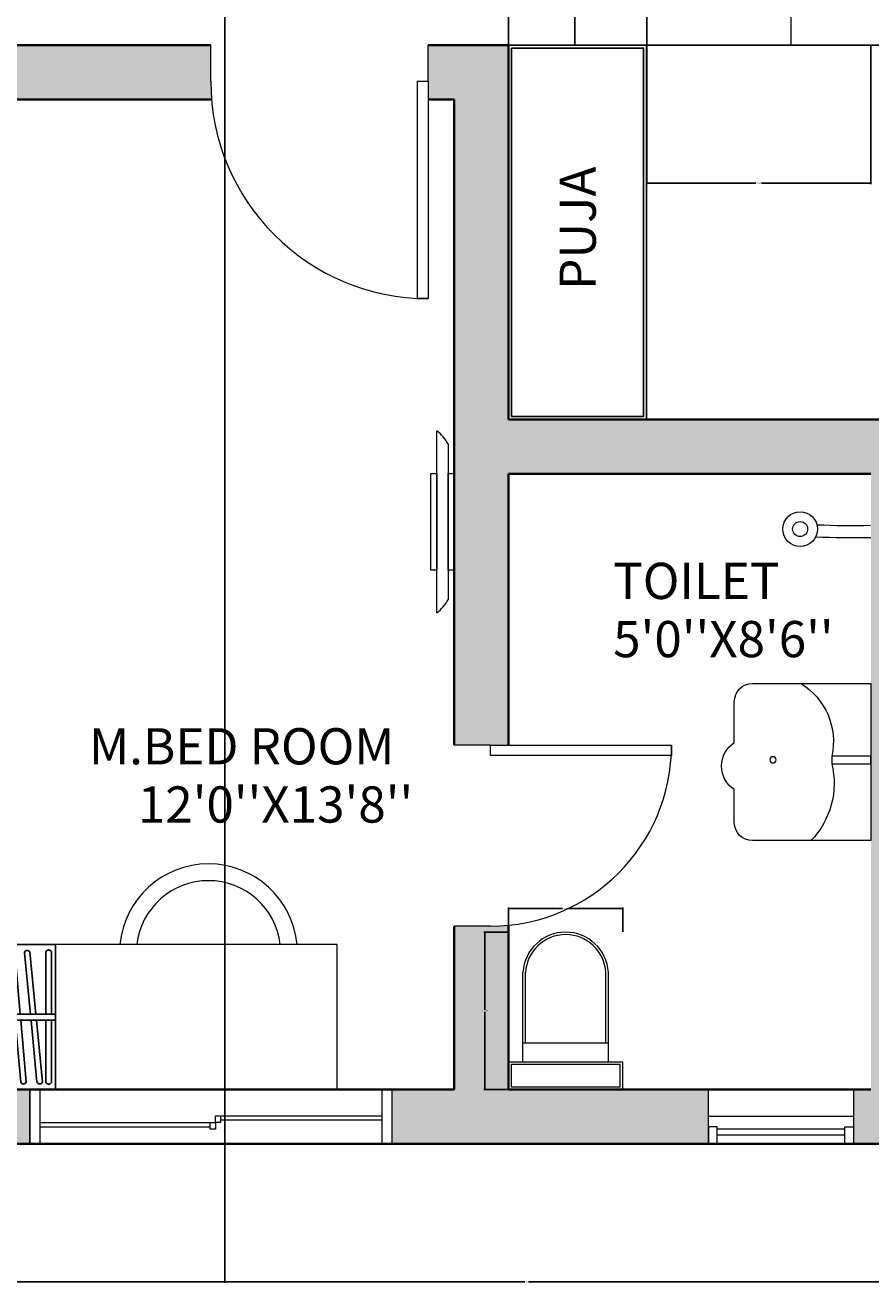
# Model space of a CAD drawing. Units: inches. Extents: x 1789 to 2841, y 3180 to 3702.
# Tile 3 of 14: x 2041 to 2181, y 3180 to 3388. Entities that reach past the tile are written whole.
import ezdxf

# ---------------------------------------------------------------- set-up
doc = ezdxf.new("R2010")
doc.units = ezdxf.units.IN
doc.header["$MEASUREMENT"] = 0
for name, color, linetype, lineweight in [('A-ANNO-DIMS', 2, 'Continuous', 18), ('A-AREA-IDEN', 7, 'Continuous', 18), ('A-EQPM', 8, 'Continuous', 18), ('A-FLOR-CASE', 34, 'Continuous', 25), ('A-FLOR-FIXT', 9, 'Continuous', 18), ('A-WALL', 40, 'Continuous', 35), ('A-WALL-PATT', 252, 'Continuous', 13), ('DORS', 70, 'Continuous', 18), ('FURNITURE', 34, 'Continuous', 18), ('WINDOWS', 130, 'Continuous', 18)]:
    doc.layers.add(name, color=color, linetype=linetype, lineweight=lineweight)
doc.styles.get("Standard").update_dxf_attribs({"font": 'arial.ttf'})
doc.dimstyles.get("Standard").update_dxf_attribs({"dimtxt": 0.18, "dimasz": 0.18, "dimexe": 0.18, "dimexo": 0.0625, "dimgap": 0.09, "dimtad": 0, "dimtih": 1, "dimtoh": 1, "dimdec": 0, "dimzin": 0, "dimdsep": 46, "dimlunit": 3, "dimtxsty": 'Standard', "dimcen": 0.09, "dimadec": 0, "dimazin": 0, "dimtfac": 1, "dimtdec": 0, "dimtofl": 0, "dimtmove": 0, "dimatfit": 3, "dimfxl": 1, "dimtolj": 1, "dimtzin": 0, "dimarcsym": 0})

# ---------------------------------------------------------------- blocks, each defined once
blk = doc.blocks.new('CUBOARD')
for p, q in [((2183.73, 3646.16), (2183.73, 3568.16)), ((2184.71, 3646.16), (2184.71, 3568.16))]:
    blk.add_line(p, q)
blk.add_lwpolyline([(2172.23, 3646.16), (2196.23, 3646.16), (2196.23, 3568.16), (2172.23, 3568.16)], close=True)
for points in [[(2183.69, 3644.46), (2173.95, 3643.51)], [(2195.39, 3645.6), (2184.67, 3644.55)], [(2184.76, 3643.66), (2195.54, 3644.71)], [(2195.78, 3645.16), (2195.78, 3645.18)], [(2183.73, 3641.98), (2173.93, 3641.98)], [(2173.97, 3642.61), (2183.78, 3643.57)], [(2195.47, 3641.98), (2184.71, 3641.98)], [(2173.86, 3641.08), (2183.73, 3641.08)], [(2183.76, 3639.46), (2173.96, 3640.08)], [(2184.71, 3641.08), (2195.53, 3641.08)], [(2195.82, 3641.5), (2195.82, 3641.53)], [(2173.84, 3639.19), (2183.7, 3638.57)], [(2184.68, 3638.5), (2195.46, 3637.81)], [(2195.45, 3638.71), (2184.74, 3639.4)], [(2195.77, 3638.22), (2195.78, 3638.24)], [(2173.83, 3635.92), (2183.73, 3635.92)], [(2183.73, 3636.82), (2173.9, 3636.82)], [(2195.43, 3636.82), (2184.71, 3636.82)], [(2184.71, 3635.92), (2195.5, 3635.92)], [(2195.78, 3636.35), (2195.78, 3636.37)], [(2173.81, 3633.34), (2183.73, 3633.34)], [(2183.73, 3634.24), (2173.88, 3634.24)], [(2195.42, 3634.24), (2184.71, 3634.24)], [(2184.71, 3633.34), (2195.48, 3633.34)], [(2195.77, 3633.77), (2195.77, 3633.79)], [(2183.73, 3631.66), (2173.86, 3631.66)], [(2195.4, 3631.66), (2184.71, 3631.66)], [(2195.75, 3631.19), (2195.75, 3631.21)], [(2173.8, 3630.76), (2183.73, 3630.76)], [(2183.73, 3629.08), (2173.85, 3629.08)], [(2184.71, 3630.76), (2195.47, 3630.76)], [(2195.38, 3629.08), (2184.71, 3629.08)], [(2173.78, 3628.19), (2183.73, 3628.19)], [(2183.8, 3626.57), (2173.93, 3627.31)], [(2184.71, 3628.19), (2195.45, 3628.19)], [(2195.73, 3628.61), (2195.73, 3628.63)], [(2173.79, 3626.43), (2183.74, 3625.68)], [(2184.71, 3625.61), (2195.4, 3624.81)], [(2195.4, 3625.7), (2184.78, 3626.5)], [(2195.72, 3625.21), (2195.72, 3625.23)], [(2173.75, 3623.03), (2183.73, 3623.03)], [(2183.73, 3623.92), (2173.81, 3623.92)], [(2195.35, 3623.92), (2184.71, 3623.92)], [(2184.71, 3623.03), (2195.42, 3623.03)], [(2195.7, 3623.45), (2195.7, 3623.48)], [(2183.73, 3621.34), (2173.8, 3621.34)], [(2195.33, 3621.34), (2184.71, 3621.34)], [(2195.68, 3620.87), (2195.68, 3620.9)], [(2173.73, 3620.45), (2183.73, 3620.45)], [(2183.67, 3618.69), (2173.75, 3617.93)], [(2195.22, 3619.57), (2184.65, 3618.76)], [(2184.71, 3620.45), (2195.4, 3620.45)], [(2184.71, 3617.87), (2195.35, 3618.68)], [(2195.6, 3619.13), (2195.6, 3619.15)], [(2173.75, 3617.03), (2183.74, 3617.8)], [(2173.7, 3615.29), (2183.73, 3615.29)], [(2183.73, 3616.19), (2173.77, 3616.19)], [(2195.3, 3616.19), (2184.71, 3616.19)], [(2184.71, 3615.29), (2195.37, 3615.29)], [(2195.65, 3615.71), (2195.65, 3615.74)], [(2173.68, 3612.71), (2183.73, 3612.71)], [(2183.73, 3613.61), (2173.75, 3613.61)], [(2195.28, 3613.61), (2184.71, 3613.61)], [(2184.71, 3612.71), (2195.35, 3612.71)], [(2195.63, 3613.14), (2195.63, 3613.16)], [(2173.67, 3611.18), (2183.69, 3610.23)], [(2183.78, 3611.12), (2173.82, 3612.07)], [(2195.26, 3610.03), (2184.75, 3611.03)], [(2183.72, 3608.42), (2173.71, 3608.13)], [(2184.67, 3610.14), (2195.24, 3609.13)], [(2195.23, 3608.76), (2184.7, 3608.45)], [(2195.56, 3609.53), (2195.57, 3609.55)], [(2195.6, 3608.3), (2195.6, 3608.32)], [(2173.66, 3607.23), (2183.75, 3607.53)], [(2184.73, 3607.55), (2195.33, 3607.87)], [(2173.63, 3604.98), (2183.73, 3604.98)], [(2183.73, 3605.87), (2173.7, 3605.87)], [(2195.23, 3605.87), (2184.71, 3605.87)], [(2184.71, 3604.98), (2195.3, 3604.98)], [(2195.58, 3605.4), (2195.58, 3605.42)], [(2173.61, 3602.4), (2183.73, 3602.4)], [(2183.73, 3603.29), (2173.68, 3603.29)], [(2195.22, 3603.29), (2184.71, 3603.29)], [(2184.71, 3602.4), (2195.28, 3602.4)], [(2195.57, 3602.82), (2195.57, 3602.84)], [(2183.73, 3600.71), (2173.67, 3600.71)], [(2195.2, 3600.71), (2184.71, 3600.71)], [(2195.55, 3600.24), (2195.55, 3600.27)], [(2173.6, 3599.82), (2183.73, 3599.82)], [(2183.73, 3598.13), (2173.65, 3598.13)], [(2184.71, 3599.82), (2195.27, 3599.82)], [(2195.18, 3598.13), (2184.71, 3598.13)], [(2173.58, 3597.24), (2183.73, 3597.24)], [(2183.77, 3595.62), (2173.68, 3596.25)], [(2184.71, 3597.24), (2195.25, 3597.24)], [(2195.53, 3597.66), (2195.53, 3597.69)], [(2173.56, 3595.36), (2183.71, 3594.72)], [(2184.69, 3594.66), (2195.19, 3594)], [(2195.18, 3594.9), (2184.74, 3595.55)], [(2195.5, 3594.4), (2195.5, 3594.43)], [(2173.55, 3592.08), (2183.73, 3592.08)], [(2183.73, 3592.98), (2173.62, 3592.98)], [(2195.15, 3592.98), (2184.71, 3592.98)], [(2184.71, 3592.08), (2195.22, 3592.08)], [(2195.5, 3592.5), (2195.5, 3592.53)], [(2173.57, 3590.49), (2183.74, 3589.59)], [(2183.73, 3590.49), (2173.72, 3591.37)], [(2195.17, 3589.47), (2184.71, 3590.4)], [(2184.71, 3589.5), (2195.16, 3588.58)], [(2183.73, 3587.82), (2173.58, 3587.82)], [(2195.12, 3587.82), (2184.71, 3587.82)], [(2195.48, 3588.97), (2195.48, 3589)], [(2173.51, 3586.92), (2183.73, 3586.92)], [(2194.84, 3586.83), (2184.58, 3585.23)], [(2184.71, 3586.92), (2195.19, 3586.92)], [(2184.71, 3584.34), (2195.04, 3585.95)], [(2195.26, 3586.41), (2195.25, 3586.44)], [(2195.47, 3587.35), (2195.47, 3587.37)], [(2183.61, 3585.08), (2173.56, 3583.51)], [(2173.63, 3582.62), (2183.75, 3584.19)], [(2173.48, 3581.77), (2183.73, 3581.77)], [(2183.73, 3582.66), (2173.55, 3582.66)], [(2195.08, 3582.66), (2184.71, 3582.66)], [(2184.71, 3581.77), (2195.15, 3581.77)], [(2195.43, 3582.19), (2195.43, 3582.21)], [(2173.46, 3579.19), (2183.73, 3579.19)], [(2183.73, 3580.08), (2173.53, 3580.08)], [(2195.07, 3580.08), (2184.71, 3580.08)], [(2184.71, 3579.19), (2195.14, 3579.19)], [(2195.42, 3579.61), (2195.42, 3579.63)], [(2183.73, 3577.5), (2173.52, 3577.5)], [(2195.05, 3577.5), (2184.71, 3577.5)], [(2195.4, 3577.03), (2195.4, 3577.05)], [(2173.45, 3576.61), (2183.73, 3576.61)], [(2194.92, 3575.81), (2184.64, 3574.92)], [(2184.71, 3576.61), (2195.12, 3576.61)], [(2184.71, 3574.03), (2195.06, 3574.93)], [(2195.31, 3575.37), (2195.31, 3575.4)], [(2183.66, 3574.84), (2173.46, 3573.95)], [(2173.47, 3573.05), (2183.74, 3573.94)], [(2194.88, 3573.34), (2184.63, 3572.34)], [(2195.28, 3572.91), (2195.27, 3572.93)], [(2183.65, 3572.24), (2173.45, 3571.25)], [(2173.47, 3570.35), (2183.74, 3571.35)], [(2184.71, 3571.45), (2195.04, 3572.46)], [(2173.4, 3568.87), (2183.73, 3568.87)], [(2183.73, 3569.77), (2173.47, 3569.77)], [(2195, 3569.77), (2184.71, 3569.77)], [(2184.71, 3568.87), (2195.07, 3568.87)], [(2195.35, 3569.29), (2195.35, 3569.32)]]:
    blk.add_lwpolyline(points)
for centre, start, end in [((2195.31, 3645.13), 7.0195, 80.386), ((2195.31, 3645.13), 299.464, 4.1032), ((2174.06, 3641.52), 105.1753, 246.0974), ((2174.12, 3643.06), 110.7367, 251.6587), ((2195.34, 3641.52), 1.4582, 74.8247), ((2174.06, 3639.62), 101.5232, 242.4452), ((2195.34, 3641.52), 293.9026, 358.5418), ((2195.3, 3638.26), 357.8061, 71.1726), ((2195.3, 3638.26), 290.2505, 354.8897), ((2174.02, 3636.36), 105.1753, 246.0974), ((2195.31, 3636.36), 1.4582, 74.8247), ((2195.31, 3636.36), 293.9026, 358.5418), ((2174.01, 3633.78), 105.1753, 246.0974), ((2195.29, 3633.78), 1.4582, 74.8247), ((2195.29, 3633.78), 293.9026, 358.5418), ((2173.99, 3631.2), 105.1753, 246.0974), ((2195.27, 3631.2), 1.4582, 74.8247), ((2195.27, 3631.2), 293.9026, 358.5418), ((2173.97, 3628.62), 105.1753, 246.0974), ((2195.26, 3628.62), 1.4582, 74.8247), ((2174.02, 3626.85), 100.888, 241.81), ((2195.26, 3628.62), 293.9026, 358.5418), ((2195.24, 3625.25), 357.1709, 70.5374), ((2195.24, 3625.25), 289.6153, 354.2545), ((2173.94, 3623.46), 105.1753, 246.0974), ((2195.22, 3623.46), 1.4582, 74.8247), ((2195.22, 3623.46), 293.9026, 358.5418), ((2173.92, 3620.88), 105.1753, 246.0974), ((2195.21, 3620.88), 1.4582, 74.8247), ((2195.21, 3620.88), 293.9026, 358.5418), ((2195.13, 3619.1), 5.8369, 79.2034), ((2195.13, 3619.1), 298.2814, 2.9206), ((2173.9, 3617.48), 109.5541, 250.4761), ((2173.89, 3615.73), 105.1753, 246.0974), ((2195.17, 3615.73), 1.4582, 74.8247), ((2195.17, 3615.73), 293.9026, 358.5418), ((2173.87, 3613.15), 105.1753, 246.0974), ((2195.16, 3613.15), 1.4582, 74.8247), ((2195.16, 3613.15), 293.9026, 358.5418), ((2173.9, 3611.6), 99.7479, 240.6699), ((2195.12, 3608.3), 3.1408, 76.5073), ((2195.09, 3609.58), 288.4752, 353.1144), ((2195.09, 3609.58), 356.0307, 69.3973), ((2195.12, 3608.3), 295.5853, 0.2245), ((2173.84, 3607.67), 106.858, 247.78), ((2173.82, 3605.41), 105.1753, 246.0974), ((2195.11, 3605.41), 1.4582, 74.8247), ((2195.11, 3605.41), 293.9026, 358.5418), ((2173.81, 3602.83), 105.1753, 246.0974), ((2195.09, 3602.83), 1.4582, 74.8247), ((2195.09, 3602.83), 293.9026, 358.5418), ((2173.79, 3600.25), 105.1753, 246.0974), ((2195.08, 3600.25), 1.4582, 74.8247), ((2195.08, 3600.25), 293.9026, 358.5418), ((2173.77, 3597.67), 105.1753, 246.0974), ((2195.06, 3597.67), 1.4582, 74.8247), ((2173.78, 3595.78), 101.566, 242.4881), ((2195.06, 3597.67), 293.9026, 358.5418), ((2195.02, 3594.44), 357.8489, 71.2154), ((2195.02, 3594.44), 290.2933, 354.9325), ((2173.74, 3592.52), 105.1753, 246.0974), ((2195.03, 3592.52), 1.4582, 74.8247), ((2195.03, 3592.52), 293.9026, 358.5418), ((2173.8, 3590.9), 100.1162, 241.0382), ((2173.71, 3587.36), 105.1753, 246.0974), ((2194.99, 3587.36), 1.4582, 74.8247), ((2195.01, 3589.03), 288.8435, 353.4827), ((2195.01, 3589.03), 356.399, 69.7655), ((2194.79, 3586.35), 10.3063, 83.6728), ((2194.79, 3586.35), 302.7507, 7.3899), ((2194.99, 3587.36), 293.9026, 358.5418), ((2173.75, 3583.08), 114.0234, 254.9455), ((2173.67, 3582.2), 105.1753, 246.0974), ((2194.96, 3582.2), 1.4582, 74.8247), ((2194.96, 3582.2), 293.9026, 358.5418), ((2173.66, 3579.62), 105.1753, 246.0974), ((2194.94, 3579.62), 1.4582, 74.8247), ((2194.94, 3579.62), 293.9026, 358.5418), ((2173.64, 3577.04), 105.1753, 246.0974), ((2194.93, 3577.04), 1.4582, 74.8247), ((2194.93, 3577.04), 293.9026, 358.5418), ((2194.83, 3575.34), 6.4142, 79.7807), ((2194.83, 3575.34), 298.8587, 3.4979), ((2173.63, 3573.5), 110.1314, 251.0534), ((2194.8, 3572.87), 7.0476, 80.4142), ((2194.8, 3572.87), 299.4921, 4.1313), ((2173.62, 3570.8), 110.7648, 251.6868), ((2173.59, 3569.31), 105.1753, 246.0974), ((2194.88, 3569.31), 1.4582, 74.8247), ((2194.88, 3569.31), 293.9026, 358.5418)]:
    blk.add_arc(centre, 0.476, start, end)
blk = doc.blocks.new('KIKI')
blk.add_lwpolyline([(2076.233, 3621.086), (2067.627, 3621.086), (2067.627, 3604.375), (2076.233, 3604.375)], close=True)
for radius, start, end in [(5.285, 95.30288, 264.69712), (4.285, 96.54542, 263.45458)]:
    blk.add_arc((2068.115, 3613.452), radius, start, end)
blk = doc.blocks.new('HYJ')
for p, q in [((2236.02, 3650.77), (2262.74, 3650.77)), ((2236.02, 3650.11), (2262.74, 3650.11)), ((2206.12, 3649.67), (2234.3, 3649.67)), ((2206.12, 3649), (2234.3, 3649))]:
    blk.add_line(p, q)
for points in [[(2204.43, 3646.16), (2264.43, 3646.16), (2264.43, 3655.16), (2204.43, 3655.16)], [(2204.43, 3655.16), (2206.12, 3655.16), (2206.12, 3646.16), (2204.43, 3646.16)], [(2264.43, 3655.16), (2262.74, 3655.16), (2262.74, 3646.16), (2264.43, 3646.16)], [(2235.16, 3650.77), (2236.02, 3650.77), (2236.02, 3649.67), (2235.16, 3649.67)], [(2234.3, 3649.67), (2235.16, 3649.67), (2235.16, 3648.56), (2234.3, 3648.56)]]:
    blk.add_lwpolyline(points, close=True)
blk = doc.blocks.new('*U9')
for p, q in [((0, 0), (0, -6)), ((36, 0), (36, -6))]:
    blk.add_line(p, q)
blk.add_lwpolyline([(0, 0), (0, 36), (1.75, 36), (1.75, 0)], close=True)
blk.add_arc((0, 0), 36, 0, 90)
blk = doc.blocks.new('GTGTG')
for points in [[(2266.82, 3646.16), (2282.82, 3646.16), (2282.82, 3645.14), (2266.82, 3645.14)], [(2266.82, 3643.29), (2282.82, 3643.29), (2282.82, 3642.27), (2266.82, 3642.27)]]:
    blk.add_lwpolyline(points, close=True)
for points in [[(2261.92, 3645.14), (2287.72, 3645.14)], [(2289.9, 3643.29), (2259.74, 3643.29)]]:
    blk.add_lwpolyline(points)
for centre, start, end in [((2265.21, 3639.05), 118.4184, 142.2436), ((2284.43, 3639.05), 37.7564, 61.5816)]:
    blk.add_arc(centre, 6.92, start, end)
blk = doc.blocks.new('*U10')
for p, q in [((0, 0), (0, -6)), ((30, 0), (30, -6))]:
    blk.add_line(p, q)
blk.add_lwpolyline([(0, 0), (0, 30), (1.75, 30), (1.75, 0)], close=True)
blk.add_arc((0, 0), 30, 0, 90)
blk = doc.blocks.new('HY')
for p, q in [((2053.67, 3653.75), (2074.8, 3653.75)), ((2053.67, 3652.75), (2074.8, 3652.75)), ((2052.23, 3650.66), (2076.23, 3650.66))]:
    blk.add_line(p, q)
for points in [[(2076.23, 3646.16), (2052.23, 3646.16), (2052.23, 3655.16), (2076.23, 3655.16)], [(2052.23, 3655.16), (2053.67, 3655.16), (2053.67, 3652.35), (2052.23, 3652.35)], [(2076.23, 3655.16), (2074.8, 3655.16), (2074.8, 3652.35), (2076.23, 3652.35)]]:
    blk.add_lwpolyline(points, close=True)
blk = doc.blocks.new('GT')
for p, q in [((2141.38, 3640.15), (2141.38, 3620.49)), ((2160.08, 3640.15), (2160.08, 3620.49)), ((2141.38, 3636.04), (2160.08, 3636.04)), ((2141.93, 3636.04), (2141.93, 3620.49)), ((2159.53, 3636.04), (2159.53, 3620.49))]:
    blk.add_line(p, q)
for points in [[(2163.23, 3646.16), (2138.23, 3646.16), (2138.23, 3640.15), (2163.23, 3640.15)], [(2162.68, 3645.61), (2138.78, 3645.61), (2138.78, 3640.7), (2162.68, 3640.7)]]:
    blk.add_lwpolyline(points, close=True)
for radius in [8.82, 9.37]:
    blk.add_arc((2150.73, 3621.09), radius, 183.6546, 356.3454)
blk = doc.blocks.new('TYTY')
for p, q in [((2104.84, 3607.68), (2085.23, 3607.68)), ((2085.23, 3607.68), (2085.23, 3581.66)), ((2107.84, 3597.9), (2107.84, 3604.68)), ((2107.84, 3584.66), (2107.84, 3590.13)), ((2085.23, 3581.66), (2104.84, 3581.66))]:
    blk.add_line(p, q)
blk.add_lwpolyline([(2085.23, 3595.66), (2091.71, 3595.66), (2091.71, 3594.41), (2085.23, 3594.41)], close=True)
blk.add_circle((2101.42, 3595.04), 0.517)
for centre, radius, start, end in [((2102.58, 3598.14), 11.14, 121.1396, 192.8397), ((2104.84, 3604.68), 3, 0, 90), ((2105.34, 3594.01), 4.62, 302.7804, 57.2196), ((2104.89, 3591.14), 13.58, 166.0641, 224.2681), ((2104.84, 3584.66), 3, 270, 0)]:
    blk.add_arc(centre, radius, start, end)
blk = doc.blocks.new('SOFA')
for p, q in [((2185.57, 3479.13), (2185.57, 3482.99)), ((2185.57, 3482.99), (2290.09, 3482.99)), ((2290.09, 3482.99), (2290.09, 3460.33)), ((2159.93, 3439.46), (2194.03, 3439.46)), ((2226.79, 3388.76), (2226.79, 3418.07)), ((2260.29, 3388.76), (2260.29, 3418.07)), ((2310.14, 3409.22), (2310.14, 3394.77))]:
    blk.add_line(p, q)
for points in [[(2168.05, 3468.75), (2193.44, 3468.75), (2193.44, 3479.13), (2168.05, 3479.13)], [(2304.69, 3457.56), (2311.21, 3457.56), (2311.21, 3434.14), (2304.69, 3434.14)], [(2227.7, 3454.8), (2263.24, 3454.8), (2263.24, 3433.45), (2227.7, 3433.45)], [(2168.05, 3410.16), (2193.44, 3410.16), (2193.44, 3385.14), (2168.05, 3385.14)], [(2296.77, 3394.77), (2311.21, 3394.77), (2311.21, 3409.22), (2296.77, 3409.22)]]:
    blk.add_lwpolyline(points, close=True)
for points in [[(2168.05, 3467.86), (2168.05, 3470.06, 0.414214), (2166.05, 3472.06), (2155.57, 3472.06), (2155.57, 3406.2), (2166.05, 3406.2, 0.414214), (2168.05, 3408.2), (2168.05, 3411.06)], [(2308.49, 3457.56), (2308.49, 3460.33), (2286.26, 3460.33, 0.414214), (2285.26, 3459.33), (2285.26, 3455.79, 0.414214), (2286.26, 3454.79), (2304.69, 3454.79)], [(2308.49, 3434.14), (2308.49, 3431.37), (2286.26, 3431.37, -0.414214), (2285.26, 3432.37), (2285.26, 3435.9, -0.414214), (2286.26, 3436.9), (2304.69, 3436.9)], [(2196.77, 3407.83), (2196.77, 3416.07, -0.414214), (2198.77, 3418.07), (2291.47, 3418.07, -0.414214), (2293.47, 3416.07), (2293.47, 3407.83)], [(2293.47, 3393.66, 0.414214), (2291.47, 3395.66), (2198.77, 3395.66, 0.414214), (2196.77, 3393.66)]]:
    blk.add_lwpolyline(points, format="xyb")
for points in [[(2159.93, 3468.75), (2192.03, 3468.75, -0.414214), (2194.03, 3466.75), (2194.03, 3412.16, -0.414214), (2192.03, 3410.16), (2159.93, 3410.16)], [(2284.53, 3460.33), (2311.21, 3460.33), (2311.21, 3431.37), (2284.53, 3431.37, -0.414214), (2282.53, 3433.37), (2282.53, 3458.33, -0.414214)], [(2197.2, 3407.83), (2196.33, 3407.83, 0.414214), (2194.33, 3405.83), (2194.33, 3388.76), (2199.2, 3388.76), (2199.2, 3405.83, 0.414214)], [(2293.91, 3407.83), (2293.04, 3407.83, 0.414214), (2291.04, 3405.83), (2291.04, 3388.76), (2295.91, 3388.76), (2295.91, 3405.83, 0.414214)]]:
    blk.add_lwpolyline(points, format="xyb", close=True)
for points in [[(2168.05, 3455.52), (2168.05, 3459.94)], [(2168.05, 3429.95), (2168.05, 3448.97)], [(2168.05, 3423.4), (2168.05, 3422.93)], [(2168.05, 3418.98), (2168.05, 3422.93)], [(2293.47, 3393.66), (2293.47, 3388.76), (2196.77, 3388.76), (2196.77, 3393.66)], [(2196.77, 3388.76), (2293.47, 3388.76)]]:
    blk.add_lwpolyline(points)
for centre, radius in [((2265.18, 3410.2), 1.89), ((2303.99, 3401.99), 5.76)]:
    blk.add_circle(centre, radius)
for points, knots in [([(2162.46, 3458.3), (2163.29, 3460.04), (2164.26, 3462.07), (2164.89, 3465.65), (2164.78, 3467.36), (2164.69, 3468.75)], [0, 0, 0, 0, 5.733795, 6.696566, 10.854822, 10.854822, 10.854822, 10.854822]), ([(2164.69, 3468.75), (2166.38, 3468.37), (2168.87, 3467.8), (2171.7, 3465.95), (2173.26, 3465.49), (2174.05, 3465.25)], [0, 0, 0, 0, 5.14676, 7.56322, 10.027291, 10.027291, 10.027291, 10.027291]), ([(2174.05, 3465.25), (2173.89, 3464.58), (2173.37, 3462.38), (2172.69, 3460.22), (2172.22, 3458.71)], [0, 0, 0, 0, 2.055182, 6.796603, 6.796603, 6.796603, 6.796603]), ([(2162.46, 3458.3), (2163.64, 3458.13), (2165.71, 3457.83), (2167.35, 3456.54), (2168.05, 3455.99)], [0, 0, 0, 0, 3.512009, 6.140853, 6.140853, 6.140853, 6.140853]), ([(2168.05, 3459.94), (2169.55, 3459.7), (2172.38, 3459.25), (2174.06, 3456.94), (2174.85, 3455.84)], [0, 0, 0, 0, 4.35123, 8.24052, 8.24052, 8.24052, 8.24052]), ([(2173.18, 3446.97), (2173.68, 3448.57), (2174.42, 3450.93), (2174.65, 3453.95), (2174.79, 3455.29), (2174.85, 3455.84)], [0, 0, 0, 0, 5.016146, 7.373936, 9.056838, 9.056838, 9.056838, 9.056838]), ([(2166.66, 3449.86), (2167.7, 3449.17), (2169.71, 3447.85), (2172.05, 3447.25), (2173.18, 3446.97)], [0, 0, 0, 0, 3.710874, 7.178588, 7.178588, 7.178588, 7.178588]), ([(2166.66, 3429.05), (2167.7, 3429.74), (2169.71, 3431.07), (2172.05, 3431.66), (2173.18, 3431.95)], [0, 0, 0, 0, 3.710874, 7.178588, 7.178588, 7.178588, 7.178588]), ([(2173.18, 3431.95), (2173.68, 3430.35), (2174.42, 3427.99), (2174.65, 3424.97), (2174.79, 3423.63), (2174.85, 3423.07)], [0, 0, 0, 0, 5.016146, 7.373936, 9.056838, 9.056838, 9.056838, 9.056838]), ([(2162.46, 3420.62), (2163.64, 3420.79), (2165.71, 3421.09), (2167.35, 3422.37), (2168.05, 3422.93)], [0, 0, 0, 0, 3.512009, 6.140853, 6.140853, 6.140853, 6.140853]), ([(2168.05, 3418.98), (2169.55, 3419.22), (2172.38, 3419.66), (2174.06, 3421.98), (2174.85, 3423.07)], [0, 0, 0, 0, 4.35123, 8.24052, 8.24052, 8.24052, 8.24052]), ([(2162.46, 3420.62), (2163.29, 3418.88), (2164.26, 3416.85), (2164.89, 3413.27), (2164.78, 3411.56), (2164.69, 3410.16)], [0, 0, 0, 0, 5.733795, 6.696566, 10.854822, 10.854822, 10.854822, 10.854822]), ([(2174.05, 3413.67), (2173.89, 3414.33), (2173.37, 3416.54), (2172.69, 3418.7), (2172.22, 3420.21)], [0, 0, 0, 0, 2.055182, 6.796603, 6.796603, 6.796603, 6.796603]), ([(2164.69, 3410.16), (2166.38, 3410.55), (2168.87, 3411.12), (2171.7, 3412.96), (2173.26, 3413.43), (2174.05, 3413.67)], [0, 0, 0, 0, 5.14676, 7.56322, 10.027291, 10.027291, 10.027291, 10.027291])]:
    blk.add_open_spline(points, degree=3, knots=knots)
for points in [[(2168.05, 3455.52), (2167.85, 3453.6), (2167.25, 3451.73), (2166.66, 3449.86)], [(2168.05, 3423.4), (2167.85, 3425.31), (2167.25, 3427.18), (2166.66, 3429.05)]]:
    blk.add_open_spline(points, degree=3)
blk = doc.blocks.new('SOUW')
for radius in [2.88, 1.24]:
    blk.add_circle((2096.93, 3622.15), radius)
for radius, start in [(130.14, 87.3378), (128.14, 87.3891)]:
    blk.add_arc((2088.3, 3493.42), radius, start, 91.3578)
blk = doc.blocks.new('*D45')
at = {"layer": 'A-ANNO-DIMS', "color": 0, "lineweight": -2, "transparency": 16777216}
for p, q in [((2121.17, 3238.23), (2117.14, 3238.23)), ((2117.32, 3238.05), (2117.32, 3225.38)), ((2117.32, 3212.34), (2117.32, 3225.01)), ((2121.17, 3212.16), (2117.14, 3212.16))]:
    blk.add_line(p, q, dxfattribs=at)
at = {"layer": 'A-ANNO-DIMS', "color": 0, "transparency": 16777216}
for points in [[(2117.29, 3238.05), (2117.35, 3238.05), (2117.32, 3238.23)], [(2117.29, 3212.34), (2117.35, 3212.34), (2117.32, 3212.16)]]:
    blk.add_solid(points, dxfattribs=at)
at = {"layer": 'Defpoints', "color": 0, "transparency": 16777216}
for p in [(2121.23, 3238.23), (2117.32, 3212.16), (2121.23, 3212.16)]:
    blk.add_point(p, dxfattribs=at)
at = {"layer": 'A-ANNO-DIMS', "color": 0, "transparency": 16777216, "insert": (2117.32, 3225.19), "char_height": 0.18, "attachment_point": 5}
blk.add_mtext('\\A1;WC 26 TYP.', dxfattribs=at)
blk = doc.blocks.new('*D46')
at = {"layer": 'A-ANNO-DIMS', "color": 0, "lineweight": -2, "transparency": 16777216}
for p, q in [((2121.23, 3238.29), (2121.23, 3242.31)), ((2121.41, 3242.13), (2130.17, 3242.13)), ((2139.97, 3242.13), (2131.21, 3242.13)), ((2140.15, 3238.29), (2140.15, 3242.31))]:
    blk.add_line(p, q, dxfattribs=at)
at = {"layer": 'A-ANNO-DIMS', "color": 0, "transparency": 16777216}
for points in [[(2121.41, 3242.16), (2121.41, 3242.1), (2121.23, 3242.13)], [(2139.97, 3242.16), (2139.97, 3242.1), (2140.15, 3242.13)]]:
    blk.add_solid(points, dxfattribs=at)
at = {"layer": 'Defpoints', "color": 0, "transparency": 16777216}
for p in [(2121.23, 3242.13), (2121.23, 3238.23), (2140.15, 3238.23)]:
    blk.add_point(p, dxfattribs=at)
at = {"layer": 'A-ANNO-DIMS', "color": 0, "transparency": 16777216, "insert": (2130.69, 3242.13), "char_height": 0.18, "attachment_point": 5}
blk.add_mtext('\\A1;19 TYP.', dxfattribs=at)
blk = doc.blocks.new('*D68')
at = {"layer": 'A-ANNO-DIMS', "color": 0, "lineweight": -2, "transparency": 16777216}
for p, q in [((2155.51, 3482.99), (2132.05, 3482.99)), ((2132.23, 3482.81), (2132.23, 3434.25)), ((2132.23, 3385.32), (2132.23, 3433.88)), ((2155.51, 3385.14), (2132.05, 3385.14))]:
    blk.add_line(p, q, dxfattribs=at)
at = {"layer": 'A-ANNO-DIMS', "color": 0, "transparency": 16777216}
for points in [[(2132.2, 3482.81), (2132.26, 3482.81), (2132.23, 3482.99)], [(2132.2, 3385.32), (2132.26, 3385.32), (2132.23, 3385.14)]]:
    blk.add_solid(points, dxfattribs=at)
at = {"layer": 'Defpoints', "color": 0, "transparency": 16777216}
for p in [(2132.23, 3482.99), (2155.57, 3482.99), (2155.57, 3385.14)]:
    blk.add_point(p, dxfattribs=at)
at = {"layer": 'A-ANNO-DIMS', "color": 0, "transparency": 16777216, "insert": (2132.23, 3434.07), "char_height": 0.18, "attachment_point": 5}
blk.add_mtext('\\A1;98', dxfattribs=at)
blk = doc.blocks.new('*D79')
at = {"layer": 'A-ANNO-DIMS', "color": 0, "lineweight": -2, "transparency": 16777216}
for p, q in [((1923.23, 3376.1), (1923.23, 3180.13)), ((2325.23, 3203.1), (2325.23, 3180.13)), ((1923.41, 3180.31), (2123.94, 3180.31)), ((2325.05, 3180.31), (2124.52, 3180.31))]:
    blk.add_line(p, q, dxfattribs=at)
at = {"layer": 'A-ANNO-DIMS', "color": 0, "transparency": 16777216}
for points in [[(1923.41, 3180.34), (1923.41, 3180.28), (1923.23, 3180.31)], [(2325.05, 3180.34), (2325.05, 3180.28), (2325.23, 3180.31)]]:
    blk.add_solid(points, dxfattribs=at)
at = {"layer": 'Defpoints', "color": 0, "transparency": 16777216}
for p in [(1923.23, 3376.16), (2325.23, 3203.16), (2325.23, 3180.31)]:
    blk.add_point(p, dxfattribs=at)
at = {"layer": 'A-ANNO-DIMS', "color": 0, "transparency": 16777216, "insert": (2124.23, 3180.31), "char_height": 0.18, "attachment_point": 5}
blk.add_mtext('\\A1;402', dxfattribs=at)
blk = doc.blocks.new('*D90')
at = {"layer": 'A-ANNO-DIMS', "color": 0, "lineweight": -2, "transparency": 16777216}
for p, q in [((2038.23, 3517.1), (2038.23, 3180.13)), ((2074.23, 3517.1), (2074.23, 3180.13)), ((2038.41, 3180.31), (2056.01, 3180.31)), ((2074.05, 3180.31), (2056.45, 3180.31))]:
    blk.add_line(p, q, dxfattribs=at)
at = {"layer": 'A-ANNO-DIMS', "color": 0, "transparency": 16777216}
for points in [[(2038.41, 3180.34), (2038.41, 3180.28), (2038.23, 3180.31)], [(2074.05, 3180.34), (2074.05, 3180.28), (2074.23, 3180.31)]]:
    blk.add_solid(points, dxfattribs=at)
at = {"layer": 'Defpoints', "color": 0, "transparency": 16777216}
for p in [(2038.23, 3517.16), (2074.23, 3517.16), (2074.23, 3180.31)]:
    blk.add_point(p, dxfattribs=at)
at = {"layer": 'A-ANNO-DIMS', "color": 0, "transparency": 16777216, "insert": (2056.23, 3180.31), "char_height": 0.18, "attachment_point": 5}
blk.add_mtext('\\A1;36', dxfattribs=at)
blk = doc.blocks.new('*D91')
at = {"layer": 'A-ANNO-DIMS', "color": 0, "lineweight": -2, "transparency": 16777216}
for p, q in [((2121.23, 3385.22), (2121.23, 3678.19)), ((2121.41, 3678.01), (2132.21, 3678.01)), ((2143.93, 3678.01), (2133.14, 3678.01)), ((2144.11, 3385.22), (2144.11, 3678.19))]:
    blk.add_line(p, q, dxfattribs=at)
at = {"layer": 'A-ANNO-DIMS', "color": 0, "transparency": 16777216}
for points in [[(2121.41, 3678.04), (2121.41, 3677.98), (2121.23, 3678.01)], [(2143.93, 3678.04), (2143.93, 3677.98), (2144.11, 3678.01)]]:
    blk.add_solid(points, dxfattribs=at)
at = {"layer": 'Defpoints', "color": 0, "transparency": 16777216}
for p in [(2144.11, 3678.01), (2121.23, 3385.16), (2144.11, 3385.16)]:
    blk.add_point(p, dxfattribs=at)
at = {"layer": 'A-ANNO-DIMS', "color": 0, "transparency": 16777216, "insert": (2132.67, 3678.01), "char_height": 0.18, "attachment_point": 5}
blk.add_mtext('\\A1;22.875', dxfattribs=at)
blk = doc.blocks.new('*D92')
at = {"layer": 'A-ANNO-DIMS', "color": 0, "lineweight": -2, "transparency": 16777216}
for p, q in [((2144.17, 3385.16), (2348.26, 3385.16)), ((2348.08, 3384.98), (2348.08, 3354.34)), ((2348.08, 3323.34), (2348.08, 3353.98)), ((2144.17, 3323.16), (2348.26, 3323.16))]:
    blk.add_line(p, q, dxfattribs=at)
at = {"layer": 'A-ANNO-DIMS', "color": 0, "transparency": 16777216}
for points in [[(2348.05, 3384.98), (2348.11, 3384.98), (2348.08, 3385.16)], [(2348.05, 3323.34), (2348.11, 3323.34), (2348.08, 3323.16)]]:
    blk.add_solid(points, dxfattribs=at)
at = {"layer": 'Defpoints', "color": 0, "transparency": 16777216}
for p in [(2144.11, 3385.16), (2348.08, 3385.16), (2144.11, 3323.16)]:
    blk.add_point(p, dxfattribs=at)
at = {"layer": 'A-ANNO-DIMS', "color": 0, "transparency": 16777216, "insert": (2348.08, 3354.16), "char_height": 0.18, "attachment_point": 5}
blk.add_mtext('\\A1;62', dxfattribs=at)
blk = doc.blocks.new('*D93')
at = {"layer": 'A-ANNO-DIMS', "color": 0, "lineweight": -2, "transparency": 16777216}
for p, q in [((2144.11, 3385.1), (2144.11, 3362.13)), ((2181.23, 3385.1), (2181.23, 3362.13)), ((2144.29, 3362.31), (2162.21, 3362.31)), ((2181.05, 3362.31), (2163.14, 3362.31))]:
    blk.add_line(p, q, dxfattribs=at)
at = {"layer": 'A-ANNO-DIMS', "color": 0, "transparency": 16777216}
for points in [[(2144.29, 3362.34), (2144.29, 3362.28), (2144.11, 3362.31)], [(2181.05, 3362.34), (2181.05, 3362.28), (2181.23, 3362.31)]]:
    blk.add_solid(points, dxfattribs=at)
at = {"layer": 'Defpoints', "color": 0, "transparency": 16777216}
for p in [(2144.11, 3385.16), (2181.23, 3385.16), (2144.11, 3362.31)]:
    blk.add_point(p, dxfattribs=at)
at = {"layer": 'A-ANNO-DIMS', "color": 0, "transparency": 16777216, "insert": (2162.67, 3362.31), "char_height": 0.18, "attachment_point": 5}
blk.add_mtext('\\A1;37.125', dxfattribs=at)
blk = doc.blocks.new('*D116')
at = {"layer": 'A-ANNO-DIMS', "color": 0, "lineweight": -2, "transparency": 16777216}
for p, q in [((1789.65, 3701.85), (1789.83, 3701.85)), ((1789.83, 3701.85), (1945.65, 3528.3)), ((2205.56, 3238.68), (2205.74, 3238.68)), ((2205.65, 3238.59), (2205.65, 3238.77))]:
    blk.add_line(p, q, dxfattribs=at)
at = {"layer": 'A-ANNO-DIMS', "color": 0, "transparency": 16777216}
blk.add_solid([(1945.67, 3528.32), (1945.62, 3528.28), (1945.77, 3528.16)], dxfattribs=at)
at = {"layer": 'Defpoints', "color": 0, "transparency": 16777216}
for p in [(1945.77, 3528.16), (2205.65, 3238.68)]:
    blk.add_point(p, dxfattribs=at)
at = {"layer": 'A-ANNO-DIMS', "color": 0, "transparency": 16777216, "insert": (1789.28, 3701.85), "char_height": 0.18, "attachment_point": 5}
blk.add_mtext('\\A1;R389', dxfattribs=at)

msp = doc.modelspace()

# ---------------------------------------------------------------- hatches: boundary and pattern name
at = {"layer": 'A-WALL-PATT'}
h = msp.add_hatch(color=256, dxfattribs=at)
h.dxf.hatch_style = 1
h.paths.add_polyline_path([(1968.2333, 3376.1608), (2072.0492, 3376.1608, -0.02086055), (2071.924, 3379.1608), (2071.924, 3385.1608), (2001.2333, 3385.1608), (2001.2333, 3413.9882), (1992.2333, 3413.9882), (1992.2333, 3385.1608), (1968.3016, 3385.1608), (1959.2333, 3385.1608), (1959.2333, 3376.1608), (1959.2333, 3260.1608), (1968.2333, 3260.1608), (1968.2333, 3275.5886), (1968.2333, 3332.3251)])
h = msp.add_hatch(color=256, dxfattribs=at)
h.dxf.hatch_style = 1
h.paths.add_polyline_path([(2213.8514, 3203.1608), (2213.8514, 3212.1608), (2190.2333, 3212.1608), (2190.2333, 3323.1608), (2121.2333, 3323.1608), (2121.2333, 3385.1608), (2107.924, 3385.1608), (2107.924, 3379.1608), (2107.924, 3376.1608), (2112.2333, 3376.1608), (2112.2333, 3269.2132), (2118.2333, 3269.2132), (2121.2333, 3269.2132), (2121.2333, 3314.1608), (2181.2333, 3314.1608), (2181.2333, 3212.1608), (2178.3707, 3212.1608), (2178.3707, 3203.1608)])
h.paths.add_polyline_path([(2050.2092, 3264.3521), (2108.2631, 3264.3521), (2108.2631, 3273.6652), (2050.2092, 3273.6652)], flags=9)
h = msp.add_hatch(color=256, dxfattribs=at)
h.dxf.hatch_style = 1
h.paths.add_polyline_path([(2154.3707, 3212.1608), (2121.2333, 3212.1608), (2121.2333, 3216.7108), (2121.2333, 3239.3636, -0.02504709), (2118.2333, 3239.2132), (2112.2333, 3239.2132), (2112.2333, 3212.1608), (2101.9504, 3212.1608), (2101.9504, 3203.1608), (2154.3707, 3203.1608)])
h.paths.add_polyline_path([(2041.9504, 3212.1608), (1968.2333, 3212.1608), (1968.2333, 3236.1608), (1959.2333, 3236.1608), (1959.2333, 3203.1608), (2041.9504, 3203.1608)])

# ---------------------------------------------------------------- linework, layer by layer
at = {"layer": 'A-FLOR-CASE'}
for points in [[(2121.2333, 3385.1608), (2144.1086, 3385.1608), (2144.1086, 3323.1608), (2121.2333, 3323.1608)], [(2121.7333, 3384.6608), (2143.6086, 3384.6608), (2143.6086, 3323.6608), (2121.7333, 3323.6608)]]:
    msp.add_lwpolyline(points, close=True, dxfattribs=at)
at = {"layer": 'A-WALL'}
for p, q in [((2001.2333, 3385.1608), (2071.924, 3385.1608)), ((2107.924, 3385.1608), (2121.2333, 3385.1608)), ((2121.2333, 3385.1608), (2121.2333, 3323.1608)), ((1968.2333, 3376.1608), (2072.0492, 3376.1608)), ((2107.924, 3376.1608), (2112.2333, 3376.1608)), ((2112.2333, 3376.1608), (2112.2333, 3269.2132)), ((2121.2333, 3323.1608), (2190.2333, 3323.1608)), ((2121.2333, 3314.1608), (2181.2333, 3314.1608)), ((2121.2333, 3314.1608), (2121.2333, 3269.2132)), ((2112.2333, 3239.2132), (2112.2333, 3212.1608)), ((2121.2333, 3239.3636), (2121.2333, 3212.1608)), ((1968.2333, 3212.1608), (2112.2333, 3212.1608)), ((2121.2333, 3212.1608), (2181.2333, 3212.1608)), ((1959.2333, 3203.1608), (2325.2333, 3203.1608))]:
    msp.add_line(p, q, dxfattribs=at)

# ---------------------------------------------------------------- block references
at = {"layer": 'A-EQPM', "rotation": 270}
msp.add_blockref('GTGTG', (-1533.9274, 5581.0033), dxfattribs=at)
at = {"layer": 'A-FLOR-CASE', "rotation": 90}
msp.add_blockref('CUBOARD', (5614.3941, 1039.9274), dxfattribs=at)
at = {"layer": 'A-FLOR-FIXT', "rotation": 180}
msp.add_blockref('SOUW', (4266.4533, 6927.1407), dxfattribs=at)
at = {"layer": 'A-FLOR-FIXT', "xscale": -1}
msp.add_blockref('TYTY', (4266.4667, -328.2819), dxfattribs=at)
at = {"layer": 'A-FLOR-FIXT', "xscale": 0.756665822373692, "yscale": 0.756665822373692, "zscale": 0.756665822373692, "rotation": 179.9999999999993}
msp.add_blockref('GT', (3758.0781, 5971.086), dxfattribs=at)
at = {"layer": 'DORS'}
for name, p, rotation in [('*U9', (2107.924, 3379.1608), 180), ('*U10', (2118.2333, 3269.2132), 270)]:
    msp.add_blockref(name, p, dxfattribs=dict(at, rotation=rotation))
at = {"layer": 'FURNITURE'}
msp.add_blockref('SOFA', (0, 0), dxfattribs=at)
at = {"layer": 'FURNITURE', "xscale": 2.788618734312648, "yscale": 2.788618734312648, "zscale": 2.788618734312648, "rotation": 270}
msp.add_blockref('KIKI', (-8004.9935, 9001.984), dxfattribs=at)
at = {"layer": 'WINDOWS'}
msp.add_blockref('HYJ', (-162.4821, -443), dxfattribs=at)
at = {"layer": 'WINDOWS', "rotation": 180}
msp.add_blockref('HY', (4230.604, 6858.3216), dxfattribs=at)

# ---------------------------------------------------------------- texts
at = {"layer": 'A-ANNO-DIMS'}
for s, p in [("5'0''X8'6''", (2138.5619, 3283.7619)), ("12'0''X13'8''", (2059.8453, 3256.3681))]:
    msp.add_text(s, height=6, dxfattribs=at).set_placement(p)
at = {"layer": 'A-AREA-IDEN'}
msp.add_text('PUJA', height=6, rotation=90, dxfattribs=at).set_placement((2135.6872, 3344.6141))
for s, p in [('TOILET', (2138.5619, 3293.4004)), ('M.BED ROOM', (2051.7614, 3266.0066))]:
    msp.add_text(s, height=6, dxfattribs=at).set_placement(p)

# ---------------------------------------------------------------- dimensions: what is measured, and where the dimension line sits
at = {"layer": 'A-ANNO-DIMS'}
dim = msp.add_radius_dim(center=(2205.6545, 3238.6823), mpoint=(1945.766, 3528.162), dimstyle='Standard', override={"dimdec": 0, "dimlfac": 1, "dimrnd": 0, "dimzin": 0, "dimdsep": 46, "dimlunit": 2}, dxfattribs=at)
dim.commit()
dim.dimension.update_dxf_attribs({"geometry": '*D116', "text_midpoint": (1789.2778, 3701.8498), "dimtype": 164})
for base, p1, p2, override, picture, middle in [((2144.1086, 3678.0108), (2121.2333, 3385.1608), (2144.1086, 3385.1608), {"dimdec": 3, "dimlfac": 1, "dimrnd": 0, "dimzin": 0, "dimdsep": 46, "dimlunit": 2}, '*D91', (2132.671, 3678.0108)), ((2074.2333, 3180.3108), (2038.2333, 3517.1608), (2074.2333, 3517.1608), {"dimdec": 0, "dimlfac": 1, "dimrnd": 0, "dimzin": 0, "dimdsep": 46, "dimlunit": 2}, '*D90', (2056.2333, 3180.3108)), ((2325.2333, 3180.3108), (1923.2333, 3376.1608), (2325.2333, 3203.1608), {"dimdec": 0, "dimlfac": 1, "dimrnd": 0, "dimzin": 0, "dimdsep": 46, "dimlunit": 2}, '*D79', (2124.2333, 3180.3108))]:
    dim = msp.add_linear_dim(base=base, p1=p1, p2=p2, dimstyle='Standard', override=override, dxfattribs=at)
    dim.commit()
    dim.dimension.update_dxf_attribs({"geometry": picture, "text_midpoint": middle})
for base, p1, p2, angle, override, picture, middle in [((2132.226, 3482.9891), (2155.5718, 3385.1441), (2155.5718, 3482.9891), 90, {"dimdec": 0, "dimlfac": 1, "dimrnd": 0, "dimzin": 0, "dimdsep": 46, "dimlunit": 2}, '*D68', (2132.226, 3434.0666)), ((2348.0833, 3385.1608), (2144.1086, 3323.1608), (2144.1086, 3385.1608), 90, {"dimdec": 0, "dimlfac": 1, "dimrnd": 0, "dimzin": 0, "dimdsep": 46, "dimlunit": 2}, '*D92', (2348.0833, 3354.1608)), ((2144.1086, 3362.3108), (2181.2333, 3385.1608), (2144.1086, 3385.1608), 180, {"dimdec": 3, "dimlfac": 1, "dimrnd": 0, "dimzin": 0, "dimdsep": 46, "dimlunit": 2}, '*D93', (2162.671, 3362.3108))]:
    dim = msp.add_linear_dim(base=base, p1=p1, p2=p2, angle=angle, dimstyle='Standard', override=override, dxfattribs=at)
    dim.commit()
    dim.dimension.update_dxf_attribs({"geometry": picture, "text_midpoint": middle})
for base, p1, p2, angle, text, picture, middle in [((2121.2333, 3242.1348), (2140.1529, 3238.2251), (2121.2333, 3238.2251), 180, '<> TYP.', '*D46', (2130.6931, 3242.1348)), ((2117.3237, 3212.1608), (2121.2333, 3238.2251), (2121.2333, 3212.1608), 270, 'WC <> TYP.', '*D45', (2117.3237, 3225.1929))]:
    dim = msp.add_linear_dim(base=base, p1=p1, p2=p2, angle=angle, text=text, dimstyle='Standard', override={"dimdec": 0, "dimlfac": 1, "dimrnd": 0, "dimzin": 0, "dimdsep": 46, "dimlunit": 2}, dxfattribs=at)
    dim.commit()
    dim.dimension.update_dxf_attribs({"geometry": picture, "text_midpoint": middle})

doc.saveas('drawing.dxf')
